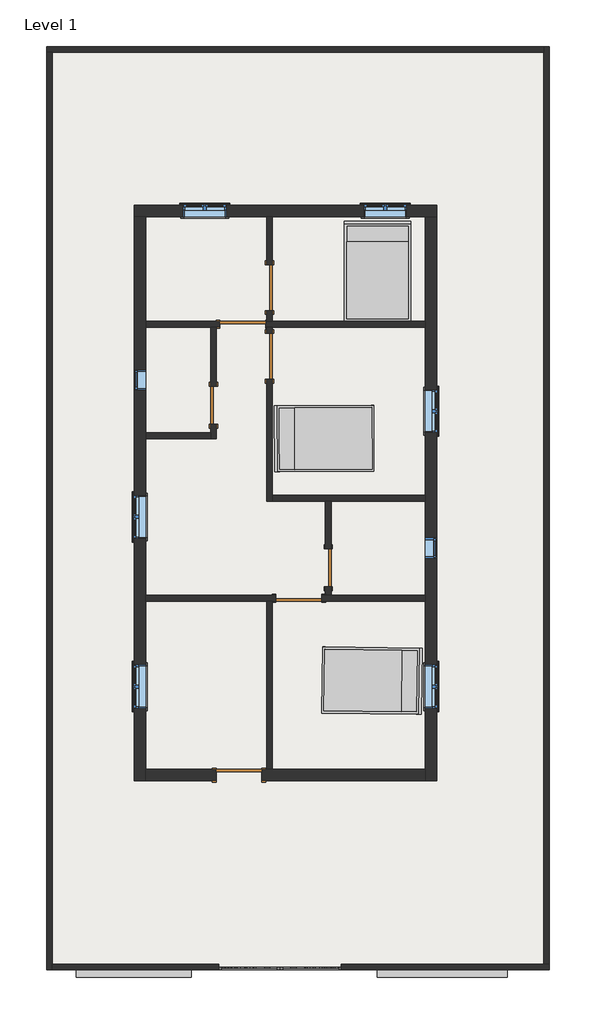
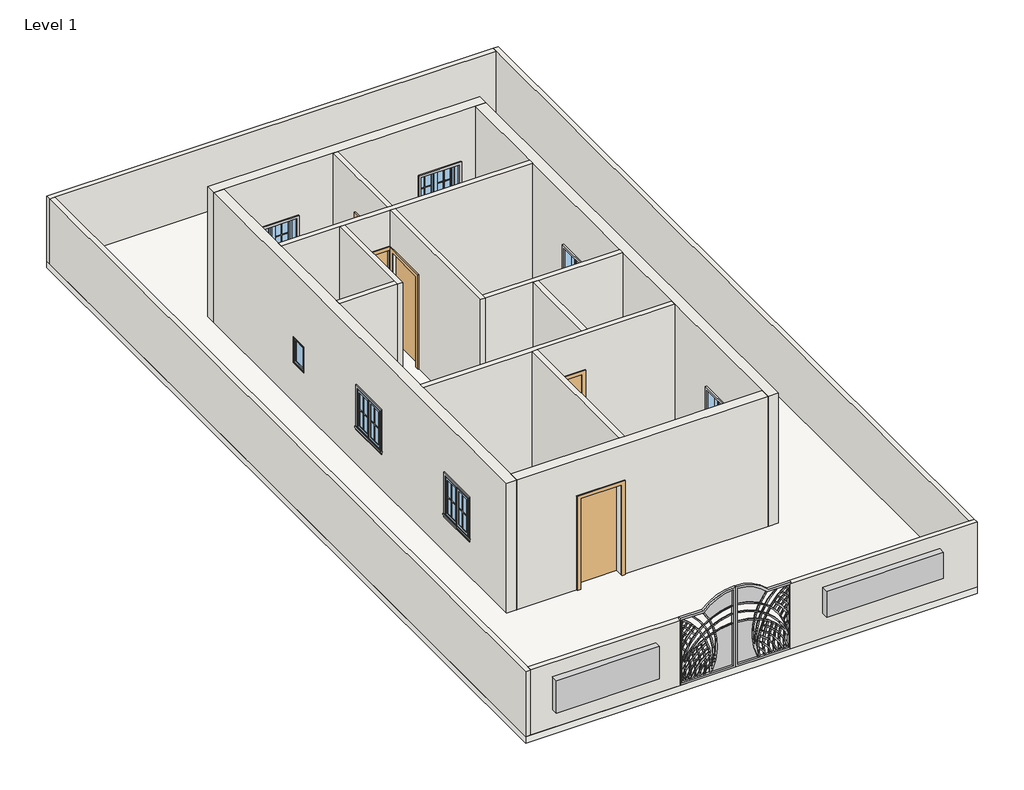
# One storey, incomplete: 26 proxies, 17 walls, 8 windows, 7 doors, 3 furniture elements, 1 slab.
"""IFC4 building model written with IfcOpenShell, lengths in millimetres."""

from ifc_helpers import new_model, si_unit, frame, origin, origin_with_axes, place, context, project, spatial, polyline, outline, extrude, faceted_brep, transform, mapped, element, save
from components import generic_models_6bc30956, generic_models_1_generic_models_1_74e75cdd, muntin_pattern_2x2_muntin_pattern_2x2_b3fe6957, muntin_pattern_2x2_muntin_pattern_2x2_3e0ecaf2, trim_window_exterior_flat_with_sill_41619996, trim_window_interior_flat_picture_frame_51c85655, door_d8f5dbb5, door_f2b275c1, door_e5f9f3c4, door_305aa2a5, door_0ca8825f, bed_17739_bed_17739_15c61121, window_aa618e30, window_339605e1

model = new_model("IFC4")

# Units and contexts
model_context = context("Model", 3, world=origin())
ifc_project = project(units=[si_unit("LENGTHUNIT", "METRE", prefix="MILLI")], contexts=[model_context])

# Site, building, storey
site = spatial("IfcSite", under=ifc_project)
building = spatial("IfcBuilding", under=site)
storey = spatial("IfcBuildingStorey", under=building, Name="Level 1", Elevation=0.0)

# Proxies
placement = place(None, origin())
generic_models_shape = generic_models_6bc30956(model_context)
element("IfcBuildingElementProxy", 1, Name="Generic Models", at=placement, inside=storey, context=model_context, shape_type="MappedRepresentation", body=[
    mapped(generic_models_shape, transform((-1369.5415084, -8760.8383207, 0.0), x_axis=(1.0, 0.0, 0.0), y_axis=(0.0, 1.0, 0.0), z_axis=(0.0, 0.0, 1.0))),
])
generic_models_1_generic_models_1_shape = generic_models_1_generic_models_1_74e75cdd(model_context)
element("IfcBuildingElementProxy", 2, Name="Generic Models 1 : Generic Models 1", ObjectType="Generic Models 1 : Generic Models 1", at=placement, inside=storey, context=model_context, shape_type="MappedRepresentation", body=[
    mapped(generic_models_1_generic_models_1_shape, transform((0.0, 0.0, 0.0), x_axis=(1.0, 0.0, 0.0), y_axis=(0.0, 1.0, 0.0), z_axis=(0.0, 0.0, 1.0))),
])
muntin_pattern_2x2_muntin_pattern_2x2_shape = muntin_pattern_2x2_muntin_pattern_2x2_b3fe6957(model_context)
element("IfcBuildingElementProxy", 3, Name="Muntin Pattern_2x2 : Muntin Pattern_2x2", ObjectType="Muntin Pattern_2x2 : Muntin Pattern_2x2", at=placement, inside=storey, context=model_context, shape_type="MappedRepresentation", body=[
    mapped(muntin_pattern_2x2_muntin_pattern_2x2_shape, transform((517.9959916, 6415.1185985, 984.25), x_axis=(1.0, 0.0, 0.0), y_axis=(0.0, 1.0, 0.0), z_axis=(0.0, 0.0, 1.0))),
])
element("IfcBuildingElementProxy", 4, Name="Muntin Pattern_2x2 : Muntin Pattern_2x2", ObjectType="Muntin Pattern_2x2 : Muntin Pattern_2x2", at=placement, inside=storey, context=model_context, shape_type="MappedRepresentation", body=[
    mapped(muntin_pattern_2x2_muntin_pattern_2x2_shape, transform((-3079.2790084, 6415.1185985, 984.25), x_axis=(1.0, 0.0, 0.0), y_axis=(0.0, 1.0, 0.0), z_axis=(0.0, 0.0, 1.0))),
])
element("IfcBuildingElementProxy", 5, Name="Muntin Pattern_2x2 : Muntin Pattern_2x2", ObjectType="Muntin Pattern_2x2 : Muntin Pattern_2x2", at=placement, inside=storey, context=model_context, shape_type="MappedRepresentation", body=[
    mapped(muntin_pattern_2x2_muntin_pattern_2x2_shape, transform((1751.4834916, 2536.8560985, 984.25), x_axis=(0.0, -1.0, 0.0), y_axis=(1.0, 0.0, 0.0), z_axis=(0.0, 0.0, 1.0))),
])
element("IfcBuildingElementProxy", 6, Name="Muntin Pattern_2x2 : Muntin Pattern_2x2", ObjectType="Muntin Pattern_2x2 : Muntin Pattern_2x2", at=placement, inside=storey, context=model_context, shape_type="MappedRepresentation", body=[
    mapped(muntin_pattern_2x2_muntin_pattern_2x2_shape, transform((-4261.9665084, 0.0310985, 984.25), x_axis=(0.0, 1.0, 0.0), y_axis=(-1.0, 0.0, 0.0), z_axis=(0.0, 0.0, 1.0))),
])
element("IfcBuildingElementProxy", 7, Name="Muntin Pattern_2x2 : Muntin Pattern_2x2", ObjectType="Muntin Pattern_2x2 : Muntin Pattern_2x2", at=placement, inside=storey, context=model_context, shape_type="MappedRepresentation", body=[
    mapped(muntin_pattern_2x2_muntin_pattern_2x2_shape, transform((-4261.9665084, -3381.3439015, 984.25), x_axis=(0.0, 1.0, 0.0), y_axis=(-1.0, 0.0, 0.0), z_axis=(0.0, 0.0, 1.0))),
])
element("IfcBuildingElementProxy", 8, Name="Muntin Pattern_2x2 : Muntin Pattern_2x2", ObjectType="Muntin Pattern_2x2 : Muntin Pattern_2x2", at=placement, inside=storey, context=model_context, shape_type="MappedRepresentation", body=[
    mapped(muntin_pattern_2x2_muntin_pattern_2x2_shape, transform((1751.4834916, -2952.7189015, 984.25), x_axis=(0.0, -1.0, 0.0), y_axis=(1.0, 0.0, 0.0), z_axis=(0.0, 0.0, 1.0))),
])
muntin_pattern_2x2_muntin_pattern_2x2_2_shape = muntin_pattern_2x2_muntin_pattern_2x2_3e0ecaf2(model_context)
element("IfcBuildingElementProxy", 9, Name="Muntin Pattern_2x2 : Muntin Pattern_2x2", ObjectType="Muntin Pattern_2x2 : Muntin Pattern_2x2", at=placement, inside=storey, context=model_context, shape_type="MappedRepresentation", body=[
    mapped(muntin_pattern_2x2_muntin_pattern_2x2_2_shape, transform((946.6209916, 6415.1185985, 984.25), x_axis=(-1.0, 0.0, 0.0), y_axis=(0.0, -1.0, 0.0), z_axis=(0.0, 0.0, 1.0))),
])
element("IfcBuildingElementProxy", 10, Name="Muntin Pattern_2x2 : Muntin Pattern_2x2", ObjectType="Muntin Pattern_2x2 : Muntin Pattern_2x2", at=placement, inside=storey, context=model_context, shape_type="MappedRepresentation", body=[
    mapped(muntin_pattern_2x2_muntin_pattern_2x2_2_shape, transform((-2650.6540084, 6415.1185985, 984.25), x_axis=(-1.0, 0.0, 0.0), y_axis=(0.0, -1.0, 0.0), z_axis=(0.0, 0.0, 1.0))),
])
element("IfcBuildingElementProxy", 11, Name="Muntin Pattern_2x2 : Muntin Pattern_2x2", ObjectType="Muntin Pattern_2x2 : Muntin Pattern_2x2", at=placement, inside=storey, context=model_context, shape_type="MappedRepresentation", body=[
    mapped(muntin_pattern_2x2_muntin_pattern_2x2_2_shape, transform((1751.4834916, 2108.2310985, 984.25), x_axis=(0.0, 1.0, 0.0), y_axis=(-1.0, 0.0, 0.0), z_axis=(0.0, 0.0, 1.0))),
])
element("IfcBuildingElementProxy", 12, Name="Muntin Pattern_2x2 : Muntin Pattern_2x2", ObjectType="Muntin Pattern_2x2 : Muntin Pattern_2x2", at=placement, inside=storey, context=model_context, shape_type="MappedRepresentation", body=[
    mapped(muntin_pattern_2x2_muntin_pattern_2x2_2_shape, transform((-4261.9665084, 428.6560985, 984.25), x_axis=(0.0, -1.0, 0.0), y_axis=(1.0, 0.0, 0.0), z_axis=(0.0, 0.0, 1.0))),
])
element("IfcBuildingElementProxy", 13, Name="Muntin Pattern_2x2 : Muntin Pattern_2x2", ObjectType="Muntin Pattern_2x2 : Muntin Pattern_2x2", at=placement, inside=storey, context=model_context, shape_type="MappedRepresentation", body=[
    mapped(muntin_pattern_2x2_muntin_pattern_2x2_2_shape, transform((-4261.9665084, -2952.7189015, 984.25), x_axis=(0.0, -1.0, 0.0), y_axis=(1.0, 0.0, 0.0), z_axis=(0.0, 0.0, 1.0))),
])
element("IfcBuildingElementProxy", 14, Name="Muntin Pattern_2x2 : Muntin Pattern_2x2", ObjectType="Muntin Pattern_2x2 : Muntin Pattern_2x2", at=placement, inside=storey, context=model_context, shape_type="MappedRepresentation", body=[
    mapped(muntin_pattern_2x2_muntin_pattern_2x2_2_shape, transform((1751.4834916, -3381.3439015, 984.25), x_axis=(0.0, 1.0, 0.0), y_axis=(-1.0, 0.0, 0.0), z_axis=(0.0, 0.0, 1.0))),
])
trim_window_exterior_flat_with_sill_shape = trim_window_exterior_flat_with_sill_41619996(model_context)
element("IfcBuildingElementProxy", 15, Name="Trim-Window-Exterior-Flat : with Sill", ObjectType="Trim-Window-Exterior-Flat : with Sill", at=placement, inside=storey, context=model_context, shape_type="MappedRepresentation", body=[
    mapped(trim_window_exterior_flat_with_sill_shape, transform((732.3084916, 6424.6435985, 1828.8), x_axis=(-1.0, 0.0, 0.0), y_axis=(0.0, 0.0, 1.0), z_axis=(0.0, 1.0, 0.0))),
])
element("IfcBuildingElementProxy", 16, Name="Trim-Window-Exterior-Flat : with Sill", ObjectType="Trim-Window-Exterior-Flat : with Sill", at=placement, inside=storey, context=model_context, shape_type="MappedRepresentation", body=[
    mapped(trim_window_exterior_flat_with_sill_shape, transform((-2864.9665084, 6424.6435985, 1828.8), x_axis=(-1.0, 0.0, 0.0), y_axis=(0.0, 0.0, 1.0), z_axis=(0.0, 1.0, 0.0))),
])
element("IfcBuildingElementProxy", 17, Name="Trim-Window-Exterior-Flat : with Sill", ObjectType="Trim-Window-Exterior-Flat : with Sill", at=placement, inside=storey, context=model_context, shape_type="MappedRepresentation", body=[
    mapped(trim_window_exterior_flat_with_sill_shape, transform((1761.0084916, 2322.5435985, 1828.8), x_axis=(0.0, 1.0, 0.0), y_axis=(0.0, 0.0, 1.0), z_axis=(1.0, 0.0, 0.0))),
])
element("IfcBuildingElementProxy", 18, Name="Trim-Window-Exterior-Flat : with Sill", ObjectType="Trim-Window-Exterior-Flat : with Sill", at=placement, inside=storey, context=model_context, shape_type="MappedRepresentation", body=[
    mapped(trim_window_exterior_flat_with_sill_shape, transform((-4271.4915084, 214.3435985, 1828.8), x_axis=(0.0, -1.0, 0.0), y_axis=(0.0, 0.0, 1.0), z_axis=(-1.0, 0.0, 0.0))),
])
element("IfcBuildingElementProxy", 19, Name="Trim-Window-Exterior-Flat : with Sill", ObjectType="Trim-Window-Exterior-Flat : with Sill", at=placement, inside=storey, context=model_context, shape_type="MappedRepresentation", body=[
    mapped(trim_window_exterior_flat_with_sill_shape, transform((-4271.4915084, -3167.0314015, 1828.8), x_axis=(0.0, -1.0, 0.0), y_axis=(0.0, 0.0, 1.0), z_axis=(-1.0, 0.0, 0.0))),
])
element("IfcBuildingElementProxy", 20, Name="Trim-Window-Exterior-Flat : with Sill", ObjectType="Trim-Window-Exterior-Flat : with Sill", at=placement, inside=storey, context=model_context, shape_type="MappedRepresentation", body=[
    mapped(trim_window_exterior_flat_with_sill_shape, transform((1761.0084916, -3167.0314015, 1828.8), x_axis=(0.0, 1.0, 0.0), y_axis=(0.0, 0.0, 1.0), z_axis=(1.0, 0.0, 0.0))),
])
trim_window_interior_flat_picture_frame_shape = trim_window_interior_flat_picture_frame_51c85655(model_context)
element("IfcBuildingElementProxy", 21, Name="Trim-Window-Interior-Flat : Picture Frame", ObjectType="Trim-Window-Interior-Flat : Picture Frame", at=placement, inside=storey, context=model_context, shape_type="MappedRepresentation", body=[
    mapped(trim_window_interior_flat_picture_frame_shape, transform((732.3084916, 6196.0435985, 1828.8), x_axis=(1.0, 0.0, 0.0), y_axis=(0.0, 0.0, 1.0), z_axis=(0.0, -1.0, 0.0))),
])
element("IfcBuildingElementProxy", 22, Name="Trim-Window-Interior-Flat : Picture Frame", ObjectType="Trim-Window-Interior-Flat : Picture Frame", at=placement, inside=storey, context=model_context, shape_type="MappedRepresentation", body=[
    mapped(trim_window_interior_flat_picture_frame_shape, transform((-2864.9665084, 6196.0435985, 1828.8), x_axis=(1.0, 0.0, 0.0), y_axis=(0.0, 0.0, 1.0), z_axis=(0.0, -1.0, 0.0))),
])
element("IfcBuildingElementProxy", 23, Name="Trim-Window-Interior-Flat : Picture Frame", ObjectType="Trim-Window-Interior-Flat : Picture Frame", at=placement, inside=storey, context=model_context, shape_type="MappedRepresentation", body=[
    mapped(trim_window_interior_flat_picture_frame_shape, transform((1532.4084916, 2322.5435985, 1828.8), x_axis=(0.0, -1.0, 0.0), y_axis=(0.0, 0.0, 1.0), z_axis=(-1.0, 0.0, 0.0))),
])
element("IfcBuildingElementProxy", 24, Name="Trim-Window-Interior-Flat : Picture Frame", ObjectType="Trim-Window-Interior-Flat : Picture Frame", at=placement, inside=storey, context=model_context, shape_type="MappedRepresentation", body=[
    mapped(trim_window_interior_flat_picture_frame_shape, transform((-4042.8915084, 214.3435985, 1828.8), x_axis=(0.0, 1.0, 0.0), y_axis=(0.0, 0.0, 1.0), z_axis=(1.0, 0.0, 0.0))),
])
element("IfcBuildingElementProxy", 25, Name="Trim-Window-Interior-Flat : Picture Frame", ObjectType="Trim-Window-Interior-Flat : Picture Frame", at=placement, inside=storey, context=model_context, shape_type="MappedRepresentation", body=[
    mapped(trim_window_interior_flat_picture_frame_shape, transform((-4042.8915084, -3167.0314015, 1828.8), x_axis=(0.0, 1.0, 0.0), y_axis=(0.0, 0.0, 1.0), z_axis=(1.0, 0.0, 0.0))),
])
element("IfcBuildingElementProxy", 26, Name="Trim-Window-Interior-Flat : Picture Frame", ObjectType="Trim-Window-Interior-Flat : Picture Frame", at=placement, inside=storey, context=model_context, shape_type="MappedRepresentation", body=[
    mapped(trim_window_interior_flat_picture_frame_shape, transform((1532.4084916, -3167.0314015, 1828.8), x_axis=(0.0, -1.0, 0.0), y_axis=(0.0, 0.0, 1.0), z_axis=(-1.0, 0.0, 0.0))),
])

# Doors
door_shape = door_d8f5dbb5(model_context)
element("IfcDoor", 27, ObjectType="Single-Flush : 30\" x 80\"", at=placement, inside=storey, context=model_context, shape_type="MappedRepresentation", body=[
    mapped(door_shape, transform((-404.3415084, -795.3064015, 0.0), x_axis=(0.0, -1.0, 0.0), y_axis=(1.0, 0.0, 0.0), z_axis=(0.0, 0.0, 1.0))),
])
door_2_shape = door_f2b275c1(model_context)
element("IfcDoor", 28, ObjectType="Single-Flush : 30\" x 80\"", at=placement, inside=storey, context=model_context, shape_type="MappedRepresentation", body=[
    mapped(door_2_shape, transform((-2690.3415084, 2443.1935985, 0.0), x_axis=(0.0, -1.0, 0.0), y_axis=(1.0, 0.0, 0.0), z_axis=(0.0, 0.0, 1.0))),
])
door_3_shape = door_e5f9f3c4(model_context)
element("IfcDoor", 29, ObjectType="Single-Flush : 36\" x 84\"", at=placement, inside=storey, context=model_context, shape_type="MappedRepresentation", body=[
    mapped(door_3_shape, transform((-2106.1415084, 4056.0935985, 0.0), x_axis=(1.0, 0.0, 0.0), y_axis=(0.0, 1.0, 0.0), z_axis=(0.0, 0.0, 1.0))),
])
element("IfcDoor", 30, ObjectType="Single-Flush : 36\" x 84\"", at=placement, inside=storey, context=model_context, shape_type="MappedRepresentation", body=[
    mapped(door_3_shape, transform((-1572.7415084, 4786.3435985, 0.0), x_axis=(0.0, -1.0, 0.0), y_axis=(1.0, 0.0, 0.0), z_axis=(0.0, 0.0, 1.0))),
])
element("IfcDoor", 31, ObjectType="Single-Flush : 36\" x 84\"", at=placement, inside=storey, context=model_context, shape_type="MappedRepresentation", body=[
    mapped(door_3_shape, transform((-988.5415084, -1404.9064015, 0.0), x_axis=(-1.0, 0.0, 0.0), y_axis=(0.0, -1.0, 0.0), z_axis=(0.0, 0.0, 1.0))),
])
door_4_shape = door_305aa2a5(model_context)
element("IfcDoor", 32, ObjectType="Single-Flush : 36\" x 84\"", at=placement, inside=storey, context=model_context, shape_type="MappedRepresentation", body=[
    mapped(door_4_shape, transform((-1572.7415084, 3414.7435985, 0.0), x_axis=(0.0, 1.0, 0.0), y_axis=(-1.0, 0.0, 0.0), z_axis=(0.0, 0.0, 1.0))),
])
door_5_shape = door_0ca8825f(model_context)
element("IfcDoor", 33, ObjectType="Single-Flush : 36\" x 84\"", at=placement, inside=storey, context=model_context, shape_type="MappedRepresentation", body=[
    mapped(door_5_shape, transform((-2182.3415084, -4929.1564015, 0.0), x_axis=(1.0, 0.0, 0.0), y_axis=(0.0, 1.0, 0.0), z_axis=(0.0, 0.0, 1.0))),
])

# Furniture
bed_17739_bed_17739_shape = bed_17739_bed_17739_15c61121(model_context)
element("IfcFurniture", 34, ObjectType="Bed_17739 : Bed_17739", at=placement, inside=storey, context=model_context, shape_type="MappedRepresentation", body=[
    mapped(bed_17739_bed_17739_shape, transform((579.9084916, 5091.1435985, 0.0), x_axis=(1.0, 0.0, 0.0), y_axis=(0.0, 1.0, 0.0), z_axis=(0.0, 0.0, 1.0))),
])
element("IfcFurniture", 35, ObjectType="Bed_17739 : Bed_17739", at=placement, inside=storey, context=model_context, shape_type="MappedRepresentation", body=[
    mapped(bed_17739_bed_17739_shape, transform((-461.4915084, 1776.4435985, 0.0), x_axis=(-0.00529598194226197, 0.9999859761893001, 0.0), y_axis=(-0.9999859761893001, -0.00529598194226197, 0.0), z_axis=(0.0, 0.0, 1.0))),
])
element("IfcFurniture", 36, ObjectType="Bed_17739 : Bed_17739", at=placement, inside=storey, context=model_context, shape_type="MappedRepresentation", body=[
    mapped(bed_17739_bed_17739_shape, transform((445.2457081, -3048.1973462, 0.0), x_axis=(-0.012781947661401841, -0.9999183075701641, 0.0), y_axis=(0.9999183075701641, -0.012781947661401841, 0.0), z_axis=(0.0, 0.0, 1.0))),
])

# Slab
element("IfcSlab", 37, ObjectType="Generic - 12\"", at=placement, inside=storey, context=model_context, shape_type="SweptSolid", body=[
    extrude(outline(polyline([(4001.9228037, 9590.6616793), (4001.9228037, -8811.6383207), (-6018.3771963, -8811.6383207), (-6018.3771963, 9590.6616793), (4001.9228037, 9590.6616793)])), frame((0.0, 0.0, -152.4), z_axis=(0.0, 0.0, 1.0), x_axis=(1.0, 0.0, 0.0)), (0.0, 0.0, 1.0), 152.4),
])

# Walls
element("IfcWall", 38, ObjectType="WALL4.5\"", at=placement, inside=storey, context=model_context, shape_type="Brep", body=[
    faceted_brep([(-1648.9415084, 3998.9435985, 2133.6), (-1648.9415084, 3998.9435985, 0.0), (-1629.8915084, 3998.9435985, 0.0), (-1515.5915084, 3998.9435985, 0.0), (1532.4084916, 3998.9435985, 0.0), (1532.4084916, 3998.9435985, 3048.0), (-1515.5915084, 3998.9435985, 3048.0), (-1629.8915084, 3998.9435985, 3048.0), (-2633.1915084, 3998.9435985, 3048.0), (-2747.4915084, 3998.9435985, 3048.0), (-4042.8915084, 3998.9435985, 3048.0), (-4042.8915084, 3998.9435985, 0.0), (-2747.4915084, 3998.9435985, 0.0), (-2633.1915084, 3998.9435985, 0.0), (-2563.3415084, 3998.9435985, 0.0), (-2563.3415084, 3998.9435985, 2133.6), (1532.4084916, 4113.2435985, 0.0), (-1515.5915084, 4113.2435985, 0.0), (-1629.8915084, 4113.2435985, 0.0), (-1648.9415084, 4113.2435985, 0.0), (-1648.9415084, 4113.2435985, 2133.6), (-2563.3415084, 4113.2435985, 2133.6), (-2563.3415084, 4113.2435985, 0.0), (-4042.8915084, 4113.2435985, 0.0), (-4042.8915084, 4113.2435985, 3048.0), (-1629.8915084, 4113.2435985, 3048.0), (-1515.5915084, 4113.2435985, 3048.0), (1532.4084916, 4113.2435985, 3048.0)], [[[0, 1, 2, 3, 4, 5, 6, 7, 8, 9, 10, 11, 12, 13, 14, 15]], [[16, 17, 18, 19, 20, 21, 22, 23, 24, 25, 26, 27]], [[4, 3, 2, 1, 19, 18, 17, 16]], [[14, 13, 12, 11, 23, 22]], [[5, 4, 16, 27]], [[11, 10, 24, 23]], [[20, 19, 1, 0]], [[21, 20, 0, 15]], [[22, 21, 15, 14]], [[10, 9, 8, 7, 6, 5, 27, 26, 25, 24]]]),
])
element("IfcWall", 39, ObjectType="WALL4.5\"", at=placement, inside=storey, context=model_context, shape_type="Brep", body=[
    faceted_brep([(-1629.8915084, 6196.0435985, 3048.0), (-1629.8915084, 6196.0435985, 0.0), (-1629.8915084, 5243.5435985, 0.0), (-1629.8915084, 5243.5435985, 2133.6), (-1629.8915084, 4329.1435985, 2133.6), (-1629.8915084, 4329.1435985, 0.0), (-1629.8915084, 4113.2435985, 0.0), (-1629.8915084, 4113.2435985, 3048.0), (-1515.5915084, 6196.0435985, 0.0), (-1515.5915084, 6196.0435985, 3048.0), (-1515.5915084, 4113.2435985, 3048.0), (-1515.5915084, 4113.2435985, 0.0), (-1515.5915084, 4329.1435985, 0.0), (-1515.5915084, 4329.1435985, 2133.6), (-1515.5915084, 5243.5435985, 2133.6), (-1515.5915084, 5243.5435985, 0.0)], [[[0, 1, 2, 3, 4, 5, 6, 7]], [[8, 9, 10, 11, 12, 13, 14, 15]], [[1, 8, 15, 2]], [[5, 12, 11, 6]], [[1, 0, 9, 8]], [[7, 6, 11, 10]], [[13, 12, 5, 4]], [[14, 13, 4, 3]], [[15, 14, 3, 2]], [[9, 0, 7, 10]]]),
    faceted_brep([(-1629.8915084, 531.8435985, 0.0), (-1629.8915084, 531.8435985, 3048.0), (-1629.8915084, 3998.9435985, 3048.0), (-1629.8915084, 3998.9435985, 0.0), (-1629.8915084, 3871.9435985, 0.0), (-1629.8915084, 3871.9435985, 2133.6), (-1629.8915084, 2957.5435985, 2133.6), (-1629.8915084, 2957.5435985, 0.0), (-1515.5915084, 531.8435985, 3048.0), (-1515.5915084, 531.8435985, 0.0), (-1515.5915084, 646.1435985, 0.0), (-1515.5915084, 2957.5435985, 0.0), (-1515.5915084, 2957.5435985, 2133.6), (-1515.5915084, 3871.9435985, 2133.6), (-1515.5915084, 3871.9435985, 0.0), (-1515.5915084, 3998.9435985, 0.0), (-1515.5915084, 3998.9435985, 3048.0), (-1515.5915084, 646.1435985, 3048.0)], [[[0, 1, 2, 3, 4, 5, 6, 7]], [[8, 9, 10, 11, 12, 13, 14, 15, 16, 17]], [[9, 0, 7, 11, 10]], [[14, 4, 3, 15]], [[3, 2, 16, 15]], [[1, 0, 9, 8]], [[5, 4, 14, 13]], [[6, 5, 13, 12]], [[7, 6, 12, 11]], [[1, 8, 17, 16, 2]]]),
])
element("IfcWall", 40, ObjectType="WALL4.5\"", at=placement, inside=storey, context=model_context, shape_type="Brep", body=[
    faceted_brep([(-1515.5915084, 531.8435985, 0.0), (-461.4915084, 531.8435985, 0.0), (-347.1915084, 531.8435985, 0.0), (1532.4084916, 531.8435985, 0.0), (1532.4084916, 531.8435985, 3048.0), (-347.1915084, 531.8435985, 3048.0), (-461.4915084, 531.8435985, 3048.0), (-1515.5915084, 531.8435985, 3048.0), (-1515.5915084, 646.1435985, 0.0), (-1515.5915084, 646.1435985, 3048.0), (1532.4084916, 646.1435985, 3048.0), (1532.4084916, 646.1435985, 0.0)], [[[0, 1, 2, 3, 4, 5, 6, 7]], [[8, 9, 10, 11]], [[3, 2, 1, 0, 8, 11]], [[0, 7, 9, 8]], [[4, 3, 11, 10]], [[7, 6, 5, 4, 10, 9]]]),
])
element("IfcWall", 41, ObjectType="WALL4.5\"", at=placement, inside=storey, context=model_context, shape_type="Brep", body=[
    faceted_brep([(-2747.4915084, 2062.1935985, 2032.0), (-2747.4915084, 2062.1935985, 0.0), (-2747.4915084, 1890.7435985, 0.0), (-2747.4915084, 1776.4435985, 0.0), (-2747.4915084, 1776.4435985, 3048.0), (-2747.4915084, 1890.7435985, 3048.0), (-2747.4915084, 3998.9435985, 3048.0), (-2747.4915084, 3998.9435985, 0.0), (-2747.4915084, 2824.1935985, 0.0), (-2747.4915084, 2824.1935985, 2032.0), (-2633.1915084, 1776.4435985, 0.0), (-2633.1915084, 2062.1935985, 0.0), (-2633.1915084, 2062.1935985, 2032.0), (-2633.1915084, 2824.1935985, 2032.0), (-2633.1915084, 2824.1935985, 0.0), (-2633.1915084, 3998.9435985, 0.0), (-2633.1915084, 3998.9435985, 3048.0), (-2633.1915084, 1776.4435985, 3048.0)], [[[0, 1, 2, 3, 4, 5, 6, 7, 8, 9]], [[10, 11, 12, 13, 14, 15, 16, 17]], [[8, 7, 15, 14]], [[3, 2, 1, 11, 10]], [[7, 6, 16, 15]], [[4, 3, 10, 17]], [[12, 11, 1, 0]], [[13, 12, 0, 9]], [[14, 13, 9, 8]], [[6, 5, 4, 17, 16]]]),
])
element("IfcWall", 42, ObjectType="WALL4.5\"", at=placement, inside=storey, context=model_context, shape_type="SweptSolid", body=[
    extrude(outline(polyline([(-2747.4915084, 1776.4435985), (-4042.8915084, 1776.4435985), (-4042.8915084, 1890.7435985), (-2747.4915084, 1890.7435985), (-2747.4915084, 1776.4435985)])), origin_with_axes(), (0.0, 0.0, 1.0), 3048.0),
])
element("IfcWall", 43, ObjectType="WALL4.5\"", at=placement, inside=storey, context=model_context, shape_type="SweptSolid", body=[
    extrude(outline(polyline([(-1176.3064015, 2032.0), (-1176.3064015, 0.0), (-1347.7564015, 0.0), (-1347.7564015, 3048.0), (531.8435985, 3048.0), (531.8435985, 0.0), (-414.3064015, 0.0), (-414.3064015, 2032.0), (-1176.3064015, 2032.0)])), frame((-461.4915084, 0.0, 0.0), z_axis=(1.0, 0.0, 0.0), x_axis=(0.0, 1.0, 0.0)), (0.0, 0.0, 1.0), 114.3),
])
element("IfcWall", 44, ObjectType="WALL4.5\"", at=placement, inside=storey, context=model_context, shape_type="Brep", body=[
    faceted_brep([(-4042.8915084, -1462.0564015, 0.0), (-1629.8915084, -1462.0564015, 0.0), (-1515.5915084, -1462.0564015, 0.0), (-1445.7415084, -1462.0564015, 0.0), (-1445.7415084, -1462.0564015, 2133.6), (-531.3415084, -1462.0564015, 2133.6), (-531.3415084, -1462.0564015, 0.0), (1532.4084916, -1462.0564015, 0.0), (1532.4084916, -1462.0564015, 3048.0), (-1515.5915084, -1462.0564015, 3048.0), (-1629.8915084, -1462.0564015, 3048.0), (-4042.8915084, -1462.0564015, 3048.0), (-1445.7415084, -1347.7564015, 2133.6), (-1445.7415084, -1347.7564015, 0.0), (-4042.8915084, -1347.7564015, 0.0), (-4042.8915084, -1347.7564015, 3048.0), (-461.4915084, -1347.7564015, 3048.0), (-347.1915084, -1347.7564015, 3048.0), (1532.4084916, -1347.7564015, 3048.0), (1532.4084916, -1347.7564015, 0.0), (-347.1915084, -1347.7564015, 0.0), (-461.4915084, -1347.7564015, 0.0), (-531.3415084, -1347.7564015, 0.0), (-531.3415084, -1347.7564015, 2133.6)], [[[0, 1, 2, 3, 4, 5, 6, 7, 8, 9, 10, 11]], [[12, 13, 14, 15, 16, 17, 18, 19, 20, 21, 22, 23]], [[14, 13, 3, 2, 1, 0]], [[22, 21, 20, 19, 7, 6]], [[8, 7, 19, 18]], [[0, 11, 15, 14]], [[4, 3, 13, 12]], [[5, 4, 12, 23]], [[6, 5, 23, 22]], [[11, 10, 9, 8, 18, 17, 16, 15]]]),
])
element("IfcWall", 45, ObjectType="WALL4.5\"", at=placement, inside=storey, context=model_context, shape_type="SweptSolid", body=[
    extrude(outline(polyline([(-1629.8915084, -4814.8564015), (-1629.8915084, -1462.0564015), (-1515.5915084, -1462.0564015), (-1515.5915084, -4814.8564015), (-1629.8915084, -4814.8564015)])), origin_with_axes(), (0.0, 0.0, 1.0), 3048.0),
])
element("IfcWall", 46, ObjectType="WALL4.5\"", at=placement, inside=storey, context=model_context, shape_type="Brep", body=[
    faceted_brep([(-6018.3771963, 9476.3616793, 0.0), (-5904.0771963, 9476.3616793, 0.0), (3887.6228037, 9476.3616793, 0.0), (3887.6228037, 9476.3616793, 1524.0), (-5904.0771963, 9476.3616793, 1524.0), (-6018.3771963, 9476.3616793, 1524.0), (-6018.3771963, 9590.6616793, 0.0), (-6018.3771963, 9590.6616793, 1524.0), (3887.6228037, 9590.6616793, 1524.0), (3887.6228037, 9590.6616793, 0.0)], [[[0, 1, 2, 3, 4, 5]], [[6, 7, 8, 9]], [[2, 1, 0, 6, 9]], [[5, 4, 3, 8, 7]], [[0, 5, 7, 6]], [[3, 2, 9, 8]]]),
])
element("IfcWall", 47, ObjectType="WALL4.5\"", at=placement, inside=storey, context=model_context, shape_type="Brep", body=[
    faceted_brep([(-5904.0771963, -8811.6383207, 0.0), (-5904.0771963, -8697.3383207, 0.0), (-5904.0771963, 9476.3616793, 0.0), (-5904.0771963, 9476.3616793, 1524.0), (-5904.0771963, -8697.3383207, 1524.0), (-5904.0771963, -8811.6383207, 1524.0), (-6018.3771963, -8811.6383207, 0.0), (-6018.3771963, -8811.6383207, 1524.0), (-6018.3771963, 9476.3616793, 1524.0), (-6018.3771963, 9476.3616793, 0.0)], [[[0, 1, 2, 3, 4, 5]], [[6, 7, 8, 9]], [[2, 1, 0, 6, 9]], [[5, 4, 3, 8, 7]], [[0, 5, 7, 6]], [[3, 2, 9, 8]]]),
])
element("IfcWall", 48, ObjectType="WALL4.5\"", at=placement, inside=storey, context=model_context, shape_type="Brep", body=[
    faceted_brep([(4001.9228037, -8697.3383207, 0.0), (3887.6228037, -8697.3383207, 0.0), (-144.6271963, -8697.3383207, 0.0), (-144.6271963, -8697.3383207, 1524.0), (3887.6228037, -8697.3383207, 1524.0), (4001.9228037, -8697.3383207, 1524.0), (4001.9228037, -8811.6383207, 0.0), (4001.9228037, -8811.6383207, 1524.0), (-144.6271963, -8811.6383207, 1524.0), (-144.6271963, -8811.6383207, 0.0)], [[[0, 1, 2, 3, 4, 5]], [[6, 7, 8, 9]], [[2, 1, 0, 6, 9]], [[3, 2, 9, 8]], [[5, 4, 3, 8, 7]], [[0, 5, 7, 6]]]),
])
element("IfcWall", 49, ObjectType="WALL4.5\"", at=placement, inside=storey, context=model_context, shape_type="Brep", body=[
    faceted_brep([(3887.6228037, 9590.6616793, 0.0), (3887.6228037, 9476.3616793, 0.0), (3887.6228037, -8697.3383207, 0.0), (3887.6228037, -8697.3383207, 1524.0), (3887.6228037, 9476.3616793, 1524.0), (3887.6228037, 9590.6616793, 1524.0), (4001.9228037, 9590.6616793, 0.0), (4001.9228037, 9590.6616793, 1524.0), (4001.9228037, -8697.3383207, 1524.0), (4001.9228037, -8697.3383207, 0.0)], [[[0, 1, 2, 3, 4, 5]], [[6, 7, 8, 9]], [[2, 1, 0, 6, 9]], [[5, 4, 3, 8, 7]], [[0, 5, 7, 6]], [[3, 2, 9, 8]]]),
])
element("IfcWall", 50, ObjectType="WALL4.5\"", at=placement, inside=storey, context=model_context, shape_type="SweptSolid", body=[
    extrude(outline(polyline([(-5904.0771963, -8697.3383207), (-2583.0271963, -8697.3383207), (-2583.0271963, -8811.6383207), (-5904.0771963, -8811.6383207), (-5904.0771963, -8697.3383207)])), origin_with_axes(), (0.0, 0.0, 1.0), 1524.0),
])
element("IfcWall", 51, ObjectType="WALL9\"", at=placement, inside=storey, context=model_context, shape_type="Brep", body=[
    faceted_brep([(-4271.4915084, 6196.0435985, 0.0), (-4042.8915084, 6196.0435985, 0.0), (-1629.8915084, 6196.0435985, 0.0), (-1515.5915084, 6196.0435985, 0.0), (1532.4084916, 6196.0435985, 0.0), (1761.0084916, 6196.0435985, 0.0), (1761.0084916, 6196.0435985, 3048.0), (1532.4084916, 6196.0435985, 3048.0), (-1515.5915084, 6196.0435985, 3048.0), (-1629.8915084, 6196.0435985, 3048.0), (-4042.8915084, 6196.0435985, 3048.0), (-4271.4915084, 6196.0435985, 3048.0), (1164.1084916, 6196.0435985, 1828.8), (1164.1084916, 6196.0435985, 914.4), (300.5084916, 6196.0435985, 914.4), (300.5084916, 6196.0435985, 1828.8), (-2433.1665084, 6196.0435985, 1828.8), (-2433.1665084, 6196.0435985, 914.4), (-3296.7665084, 6196.0435985, 914.4), (-3296.7665084, 6196.0435985, 1828.8), (-4271.4915084, 6424.6435985, 0.0), (-4271.4915084, 6424.6435985, 3048.0), (1761.0084916, 6424.6435985, 3048.0), (1761.0084916, 6424.6435985, 0.0), (1164.1084916, 6424.6435985, 1828.8), (300.5084916, 6424.6435985, 1828.8), (300.5084916, 6424.6435985, 914.4), (1164.1084916, 6424.6435985, 914.4), (-2433.1665084, 6424.6435985, 1828.8), (-3296.7665084, 6424.6435985, 1828.8), (-3296.7665084, 6424.6435985, 914.4), (-2433.1665084, 6424.6435985, 914.4)], [[[0, 1, 2, 3, 4, 5, 6, 7, 8, 9, 10, 11], [12, 13, 14, 15], [16, 17, 18, 19]], [[20, 21, 22, 23], [24, 25, 26, 27], [28, 29, 30, 31]], [[5, 4, 3, 2, 1, 0, 20, 23]], [[6, 5, 23, 22]], [[0, 11, 21, 20]], [[13, 12, 24, 27]], [[14, 13, 27, 26]], [[15, 14, 26, 25]], [[12, 15, 25, 24]], [[17, 16, 28, 31]], [[18, 17, 31, 30]], [[19, 18, 30, 29]], [[16, 19, 29, 28]], [[11, 10, 9, 8, 7, 6, 22, 21]]]),
])
element("IfcWall", 52, ObjectType="WALL9\"", at=placement, inside=storey, context=model_context, shape_type="Brep", body=[
    faceted_brep([(1532.4084916, 6196.0435985, 0.0), (1532.4084916, 4113.2435985, 0.0), (1532.4084916, 3998.9435985, 0.0), (1532.4084916, 646.1435985, 0.0), (1532.4084916, 531.8435985, 0.0), (1532.4084916, -1347.7564015, 0.0), (1532.4084916, -1462.0564015, 0.0), (1532.4084916, -4814.8564015, 0.0), (1532.4084916, -5043.4564015, 0.0), (1532.4084916, -5043.4564015, 3048.0), (1532.4084916, -4814.8564015, 3048.0), (1532.4084916, -1462.0564015, 3048.0), (1532.4084916, -1347.7564015, 3048.0), (1532.4084916, 531.8435985, 3048.0), (1532.4084916, 646.1435985, 3048.0), (1532.4084916, 3998.9435985, 3048.0), (1532.4084916, 4113.2435985, 3048.0), (1532.4084916, 6196.0435985, 3048.0), (1532.4084916, -611.1564015, 1524.0), (1532.4084916, -611.1564015, 914.4), (1532.4084916, -204.7564015, 914.4), (1532.4084916, -204.7564015, 1524.0), (1532.4084916, 1890.7435985, 1828.8), (1532.4084916, 1890.7435985, 914.4), (1532.4084916, 2754.3435985, 914.4), (1532.4084916, 2754.3435985, 1828.8), (1532.4084916, -3598.8314015, 1828.8), (1532.4084916, -3598.8314015, 914.4), (1532.4084916, -2735.2314015, 914.4), (1532.4084916, -2735.2314015, 1828.8), (1761.0084916, 6196.0435985, 0.0), (1761.0084916, 6196.0435985, 3048.0), (1761.0084916, -5043.4564015, 3048.0), (1761.0084916, -5043.4564015, 0.0), (1761.0084916, -611.1564015, 1524.0), (1761.0084916, -204.7564015, 1524.0), (1761.0084916, -204.7564015, 914.4), (1761.0084916, -611.1564015, 914.4), (1761.0084916, 1890.7435985, 1828.8), (1761.0084916, 2754.3435985, 1828.8), (1761.0084916, 2754.3435985, 914.4), (1761.0084916, 1890.7435985, 914.4), (1761.0084916, -3598.8314015, 1828.8), (1761.0084916, -2735.2314015, 1828.8), (1761.0084916, -2735.2314015, 914.4), (1761.0084916, -3598.8314015, 914.4)], [[[0, 1, 2, 3, 4, 5, 6, 7, 8, 9, 10, 11, 12, 13, 14, 15, 16, 17], [18, 19, 20, 21], [22, 23, 24, 25], [26, 27, 28, 29]], [[30, 31, 32, 33], [34, 35, 36, 37], [38, 39, 40, 41], [42, 43, 44, 45]], [[8, 7, 6, 5, 4, 3, 2, 1, 0, 30, 33]], [[0, 17, 31, 30]], [[9, 8, 33, 32]], [[19, 18, 34, 37]], [[20, 19, 37, 36]], [[21, 20, 36, 35]], [[18, 21, 35, 34]], [[23, 22, 38, 41]], [[24, 23, 41, 40]], [[25, 24, 40, 39]], [[22, 25, 39, 38]], [[27, 26, 42, 45]], [[28, 27, 45, 44]], [[29, 28, 44, 43]], [[26, 29, 43, 42]], [[17, 16, 15, 14, 13, 12, 11, 10, 9, 32, 31]]]),
])
element("IfcWall", 53, ObjectType="WALL9\"", at=placement, inside=storey, context=model_context, shape_type="Brep", body=[
    faceted_brep([(-4271.4915084, 6196.0435985, 0.0), (-4271.4915084, -5043.4564015, 0.0), (-4271.4915084, -5043.4564015, 3048.0), (-4271.4915084, 6196.0435985, 3048.0), (-4271.4915084, 3148.0435985, 1524.0), (-4271.4915084, 2741.6435985, 1524.0), (-4271.4915084, 2741.6435985, 914.4), (-4271.4915084, 3148.0435985, 914.4), (-4271.4915084, 646.1435985, 1828.8), (-4271.4915084, -217.4564015, 1828.8), (-4271.4915084, -217.4564015, 914.4), (-4271.4915084, 646.1435985, 914.4), (-4271.4915084, -2735.2314015, 1828.8), (-4271.4915084, -3598.8314015, 1828.8), (-4271.4915084, -3598.8314015, 914.4), (-4271.4915084, -2735.2314015, 914.4), (-4042.8915084, 6196.0435985, 0.0), (-4042.8915084, 6196.0435985, 3048.0), (-4042.8915084, 4113.2435985, 3048.0), (-4042.8915084, 3998.9435985, 3048.0), (-4042.8915084, 1890.7435985, 3048.0), (-4042.8915084, 1776.4435985, 3048.0), (-4042.8915084, -1347.7564015, 3048.0), (-4042.8915084, -1462.0564015, 3048.0), (-4042.8915084, -4814.8564015, 3048.0), (-4042.8915084, -5043.4564015, 3048.0), (-4042.8915084, -5043.4564015, 0.0), (-4042.8915084, -4814.8564015, 0.0), (-4042.8915084, -1462.0564015, 0.0), (-4042.8915084, -1347.7564015, 0.0), (-4042.8915084, 1776.4435985, 0.0), (-4042.8915084, 1890.7435985, 0.0), (-4042.8915084, 3998.9435985, 0.0), (-4042.8915084, 4113.2435985, 0.0), (-4042.8915084, 3148.0435985, 1524.0), (-4042.8915084, 3148.0435985, 914.4), (-4042.8915084, 2741.6435985, 914.4), (-4042.8915084, 2741.6435985, 1524.0), (-4042.8915084, 646.1435985, 1828.8), (-4042.8915084, 646.1435985, 914.4), (-4042.8915084, -217.4564015, 914.4), (-4042.8915084, -217.4564015, 1828.8), (-4042.8915084, -2735.2314015, 1828.8), (-4042.8915084, -2735.2314015, 914.4), (-4042.8915084, -3598.8314015, 914.4), (-4042.8915084, -3598.8314015, 1828.8)], [[[0, 1, 2, 3], [4, 5, 6, 7], [8, 9, 10, 11], [12, 13, 14, 15]], [[16, 17, 18, 19, 20, 21, 22, 23, 24, 25, 26, 27, 28, 29, 30, 31, 32, 33], [34, 35, 36, 37], [38, 39, 40, 41], [42, 43, 44, 45]], [[1, 0, 16, 33, 32, 31, 30, 29, 28, 27, 26]], [[0, 3, 17, 16]], [[2, 1, 26, 25]], [[35, 34, 4, 7]], [[36, 35, 7, 6]], [[37, 36, 6, 5]], [[34, 37, 5, 4]], [[39, 38, 8, 11]], [[40, 39, 11, 10]], [[41, 40, 10, 9]], [[38, 41, 9, 8]], [[43, 42, 12, 15]], [[44, 43, 15, 14]], [[45, 44, 14, 13]], [[42, 45, 13, 12]], [[3, 2, 25, 24, 23, 22, 21, 20, 19, 18, 17]]]),
])
element("IfcWall", 54, ObjectType="WALL9\"", at=placement, inside=storey, context=model_context, shape_type="Brep", body=[
    faceted_brep([(-1725.1415084, -5043.4564015, 2133.6), (-1725.1415084, -5043.4564015, 0.0), (1532.4084916, -5043.4564015, 0.0), (1532.4084916, -5043.4564015, 3048.0), (-4042.8915084, -5043.4564015, 3048.0), (-4042.8915084, -5043.4564015, 0.0), (-2639.5415084, -5043.4564015, 0.0), (-2639.5415084, -5043.4564015, 2133.6), (1532.4084916, -4814.8564015, 0.0), (-1515.5915084, -4814.8564015, 0.0), (-1629.8915084, -4814.8564015, 0.0), (-1725.1415084, -4814.8564015, 0.0), (-1725.1415084, -4814.8564015, 2133.6), (-2639.5415084, -4814.8564015, 2133.6), (-2639.5415084, -4814.8564015, 0.0), (-4042.8915084, -4814.8564015, 0.0), (-4042.8915084, -4814.8564015, 3048.0), (-1629.8915084, -4814.8564015, 3048.0), (-1515.5915084, -4814.8564015, 3048.0), (1532.4084916, -4814.8564015, 3048.0)], [[[0, 1, 2, 3, 4, 5, 6, 7]], [[8, 9, 10, 11, 12, 13, 14, 15, 16, 17, 18, 19]], [[6, 5, 15, 14]], [[2, 1, 11, 10, 9, 8]], [[3, 2, 8, 19]], [[5, 4, 16, 15]], [[12, 11, 1, 0]], [[13, 12, 0, 7]], [[14, 13, 7, 6]], [[4, 3, 19, 18, 17, 16]]]),
])

# Windows
window_shape = window_aa618e30(model_context)
element("IfcWindow", 55, ObjectType="Fixed : 16\" x 24\"", at=placement, inside=storey, context=model_context, shape_type="MappedRepresentation", body=[
    mapped(window_shape, transform((1646.7084916, -446.0564015, 0.0), x_axis=(0.0, -1.0, 0.0), y_axis=(1.0, 0.0, 0.0), z_axis=(0.0, 0.0, 1.0))),
])
element("IfcWindow", 56, ObjectType="Fixed : 16\" x 24\"", at=placement, inside=storey, context=model_context, shape_type="MappedRepresentation", body=[
    mapped(window_shape, transform((-4157.1915084, 2982.9435985, 0.0), x_axis=(0.0, 1.0, 0.0), y_axis=(-1.0, 0.0, 0.0), z_axis=(0.0, 0.0, 1.0))),
])
window_2_shape = window_339605e1(model_context)
element("IfcWindow", 57, ObjectType="Window-Casement-Double : 34\" x 36\"", at=placement, inside=storey, context=model_context, shape_type="MappedRepresentation", body=[
    mapped(window_2_shape, transform((732.3084916, 6310.3435985, 0.0), x_axis=(1.0, 0.0, 0.0), y_axis=(0.0, 1.0, 0.0), z_axis=(0.0, 0.0, 1.0))),
])
element("IfcWindow", 58, ObjectType="Window-Casement-Double : 34\" x 36\"", at=placement, inside=storey, context=model_context, shape_type="MappedRepresentation", body=[
    mapped(window_2_shape, transform((-2864.9665084, 6310.3435985, 0.0), x_axis=(1.0, 0.0, 0.0), y_axis=(0.0, 1.0, 0.0), z_axis=(0.0, 0.0, 1.0))),
])
element("IfcWindow", 59, ObjectType="Window-Casement-Double : 34\" x 36\"", at=placement, inside=storey, context=model_context, shape_type="MappedRepresentation", body=[
    mapped(window_2_shape, transform((1646.7084916, 2322.5435985, 0.0), x_axis=(0.0, -1.0, 0.0), y_axis=(1.0, 0.0, 0.0), z_axis=(0.0, 0.0, 1.0))),
])
element("IfcWindow", 60, ObjectType="Window-Casement-Double : 34\" x 36\"", at=placement, inside=storey, context=model_context, shape_type="MappedRepresentation", body=[
    mapped(window_2_shape, transform((-4157.1915084, 214.3435985, 0.0), x_axis=(0.0, 1.0, 0.0), y_axis=(-1.0, 0.0, 0.0), z_axis=(0.0, 0.0, 1.0))),
])
element("IfcWindow", 61, ObjectType="Window-Casement-Double : 34\" x 36\"", at=placement, inside=storey, context=model_context, shape_type="MappedRepresentation", body=[
    mapped(window_2_shape, transform((-4157.1915084, -3167.0314015, 0.0), x_axis=(0.0, 1.0, 0.0), y_axis=(-1.0, 0.0, 0.0), z_axis=(0.0, 0.0, 1.0))),
])
element("IfcWindow", 62, ObjectType="Window-Casement-Double : 34\" x 36\"", at=placement, inside=storey, context=model_context, shape_type="MappedRepresentation", body=[
    mapped(window_2_shape, transform((1646.7084916, -3167.0314015, 0.0), x_axis=(0.0, -1.0, 0.0), y_axis=(1.0, 0.0, 0.0), z_axis=(0.0, 0.0, 1.0))),
])

save(model, "model.ifc")

# Revit data of these elements
# Type
#   m.s. sheet = none
#   2" x2" pipe = none
#   1"x1"pipe = none
#   Default Elevation = 0
# Type "Muntin Pattern_2x2 : Muntin Pattern_2x2"
#   Width [instance default] = 4' - 0"
#   Thickness = 0' - 0 1/2"
#   Height [instance default] = 4' - 0"
#   Distance = 0' - 0 3/4"
#   Interior Material [instance default] = none
#   Exterior Material [instance default] = none
#   Default Elevation = 0
# Type "Trim-Window-Exterior-Flat : with Sill"
#   Trim Width = 0' - 2 1/4"
#   Trim Thickness_Picture Frame = 0' - 1 1/4"
#   Trim Thickness_with Sill = 0' - 0 3/4"
#   Sill Thickness = 0' - 1 1/4"
#   Opening Width [instance default] = 2' - 0"
#   Opening Height [instance default] = 3' - 0"
#   Default Elevation = 4' - 0"
#   Sill = yes
#   Picture Frame = no
#   Trim Material [instance default] = none
# Type "Trim-Window-Interior-Flat : Picture Frame"
#   Trim Thickness_Picture Frame = 0' - 1 1/4"
#   Trim Width = 0' - 2 1/4"
#   Trim Thickness_with Sill = 0' - 0 3/4"
#   Sill Thickness = 0' - 1 1/4"
#   Opening Width [instance default] = 2' - 0"
#   Opening Height [instance default] = 3' - 0"
#   Default Elevation = 4' - 0"
#   Sill = no
#   Picture Frame = yes
#   Trim Material [instance default] = none
# Type "Single-Flush : 30\" x 80\""
#   Type Mark = "5"
#   Construction Type Id = "MDOOR"
#   Assembly Code = "C1020"
#   Analytic Construction = "Metal"
#   Thickness = 0' - 2"
#   Heat Transfer Coefficient (U) = 0.651978 BTU/(h·ft²·°F)
#   Height = 6' - 8"
#   Trim Projection Ext = 0' - 1"
#   Trim Projection Int = 0' - 1"
#   Trim Width = 0' - 3"
#   Width = 2' - 6"
#   Define Thermal Properties by = 1
#   Define Thermal Properties by = 1
#   Door Material = Door - Panel
#   Frame Material = Door - Frame
#   Visual Light Transmittance = 0
#   Solar Heat Gain Coefficient = 0
#   Function = (empty or 0)
#   Wall Closure = (empty or 0)
# Type "Single-Flush : 36\" x 84\""
#   Type Mark = "1"
#   Construction Type Id = "MDOOR"
#   Assembly Code = "C1020"
#   Analytic Construction = "Metal"
#   Thickness = 0' - 2"
#   Heat Transfer Coefficient (U) = 0.651978 BTU/(h·ft²·°F)
#   Height = 7' - 0"
#   Trim Projection Ext = 0' - 1"
#   Trim Projection Int = 0' - 1"
#   Trim Width = 0' - 3"
#   Width = 3' - 0"
#   Define Thermal Properties by = 1
#   Define Thermal Properties by = 1
#   Door Material = Door - Panel
#   Frame Material = Door - Frame
#   Visual Light Transmittance = 0
#   Solar Heat Gain Coefficient = 0
#   Function = (empty or 0)
#   Wall Closure = (empty or 0)
# Type "Bed_17739 : Bed_17739"
#   Default Elevation = 0
# Type "Generic - 12\""
#   Assembly Code = "B1010"
#   Function = 0
#   Layers, outside or top first: 0' - 6" no material (function 1)
# Type "WALL4.5\""
#   Assembly Code = "B2010"
#   Layers, outside or top first: 0' - 4 1/2" no material (function 1)
# Type "WALL9\""
#   Assembly Code = "B2010"
#   Layers, outside or top first: 0' - 9" no material (function 1)
# Type "Fixed : 16\" x 24\""
#   Type Mark = "4"
#   Construction Type Id = "GSP4R"
#   Assembly Code = "B2020100"
#   Analytic Construction = "1/8 in Pilkington single glazing"
#   Visual Light Transmittance = 0.9
#   Solar Heat Gain Coefficient = 0.78
#   Heat Transfer Coefficient (U) = 0.6496 BTU/(h·ft²·°F)
#   Height = 2' - 0"
#   Default Sill Height = 3' - 0"
#   Width = 1' - 4"
#   Window Inset = 0' - 0 3/4"
#   Define Thermal Properties by = 1
#   Define Thermal Properties by = 1
#   Glass Pane Material = Glass
#   Sash Material = Sash
#   Wall Closure = (empty or 0)
# Type "Window-Casement-Double : 34\" x 36\""
#   Type Mark = "14"
#   Fire Rating = "0.5h"
#   Assembly Code = "B2020100"
#   Analytic Construction = "Double glazing - domestic"
#   Frame Extension [instance default] = 0' - 0 1/4"
#   Window Inset [instance default] = 0' - 0"
#   Wall Thickness [instance default] = 0' - 6"
#   Interior Wall Closure [instance default] = 0' - 2 1/4"
#   Half Width = 1' - 5"
#   Visual Light Transmittance = 0.81
#   Thermal Resistance (R) = 1.8146 (h·ft²·°F)/BTU
#   Solar Heat Gain Coefficient = 0.76
#   Rough Width = 2' - 10 1/2"
#   Rough Height = 3' - 0 1/2"
#   Height = 3' - 0"
#   Heat Transfer Coefficient (U) = 0.5511 BTU/(h·ft²·°F)
#   Exterior Wall Closure [instance default] = 0' - 1 1/4"
#   Extension Jamb [instance default] = 0' - 2 1/4"
#   Default Sill Height = 3' - 0"
#   Width = 2' - 10"
#   Define Thermal Properties by = 0
#   Muntin Visibility = yes
#   Interior Trim Visibility [instance default] = yes
#   Exterior Trim Visibility [instance default] = yes
#   Extension Jamb Visibility [instance default] = yes
#   Interior Trim Material = Wood - Stained
#   Muntin Pattern = Muntin Pattern_2x2 : Muntin Pattern_2x2
#   Interior Trim = Trim-Window-Interior-Flat : Picture Frame
#   Interior Frame Material = Wood - Stained
#   Glass Panel Material = Glass
#   Exterior Trim Material = Clad - White
#   Exterior Trim = Trim-Window-Exterior-Flat : with Sill
#   Exterior Frame Material = Clad - White
#   Wall Closure = (empty or 0)
# Element 1 (IfcBuildingElementProxy)
#   Phase Created = New Construction
#   Materials on its faces: "r1"
# Element 2 (IfcBuildingElementProxy, "Generic Models 1 : Generic Models 1")
#   Phase Created = New Construction
#   Materials on its faces: "Blanket"
# Elements 3, 4, 5, 6, 7, 8, 9, 10, 11, 12, 13, 14 (IfcBuildingElementProxy, "Muntin Pattern_2x2 : Muntin Pattern_2x2")
#   Width = 0' - 11 5/8"
#   Height = 2' - 6 1/2"
#   Interior Material = Wood - Stained
#   Exterior Material = Clad - White
#   Phase Created = New Construction
#   Materials on its faces: "Clad - White", "Wood - Stained"
# Elements 15, 16, 17, 18, 19, 20 (IfcBuildingElementProxy, "Trim-Window-Exterior-Flat : with Sill")
#   Opening Width = 2' - 10"
#   Opening Height = 3' - 0"
#   Trim Material = Clad - White
#   Phase Created = New Construction
#   Materials on its faces: "Clad - White"
# Elements 21, 22, 23, 24, 25, 26 (IfcBuildingElementProxy, "Trim-Window-Interior-Flat : Picture Frame")
#   Opening Width = 2' - 10"
#   Opening Height = 3' - 0"
#   Trim Material = Wood - Stained
#   Phase Created = New Construction
#   Materials on its faces: "Wood - Stained"
# Elements 27, 28 (IfcDoor, "Single-Flush : 30\" x 80\"")
#   Phase Created = New Construction
#   Materials on its faces: "Door - Frame", "Door - Panel"
# Elements 29, 30, 31, 32, 33 (IfcDoor, "Single-Flush : 36\" x 84\"")
#   Phase Created = New Construction
#   Materials on its faces: "Door - Frame", "Door - Panel"
# Elements 34, 35, 36 (IfcFurniture, "Bed_17739 : Bed_17739")
#   Phase Created = New Construction
#   Materials on its faces: "legs", "sheets", "bed frame", "Blanket"
# Element 37 (IfcSlab, "Generic - 12\"")
#   Height Offset From Level = 0' - 0"
#   Phase Created = New Construction
#   Materials on its faces: "Default Floor", "Clad - White"
# Elements 38, 39, 40, 41, 42, 43, 44, 45 (IfcWall, "WALL4.5\"")
#   Top Offset = 0' - 0"
#   Base Offset = 0' - 0"
#   Unconnected Height = 10' - 0"
#   wall height = 10' - 0"
#   Phase Created = New Construction
#   Base Constraint = Level 1
#   Materials on its faces: "Default Wall"
# Elements 46, 47, 48, 49, 50 (IfcWall, "WALL4.5\"")
#   Top Offset = 0' - 0"
#   Base Offset = 0' - 0"
#   Unconnected Height = 5' - 0"
#   wall height = 5' - 0"
#   Phase Created = New Construction
#   Base Constraint = Level 1
#   Materials on its faces: "Default Wall", "Clad - White"
# Elements 51, 52, 53, 54 (IfcWall, "WALL9\"")
#   Top Offset = 0' - 0"
#   Base Offset = 0' - 0"
#   Unconnected Height = 10' - 0"
#   wall height = 10' - 0"
#   Phase Created = New Construction
#   Base Constraint = Level 1
#   Materials on its faces: "Default Wall", "Brick, Common"
# Element 55 (IfcWindow, "Fixed : 16\" x 24\"")
#   Mark = "1"
#   Phase Created = New Construction
#   Materials on its faces: "Sash", "Glass"
# Element 56 (IfcWindow, "Fixed : 16\" x 24\"")
#   Mark = "2"
#   Phase Created = New Construction
#   Materials on its faces: "Sash", "Glass"
# Element 57 (IfcWindow, "Window-Casement-Double : 34\" x 36\"")
#   Mark = "3"
#   Window Inset = 0' - 0"
#   Interior Wall Closure = 0' - 2 1/4"
#   Frame Extension = 0' - 0 1/4"
#   Exterior Wall Closure = 0' - 1 1/4"
#   Interior Trim Visibility = yes
#   Exterior Trim Visibility = yes
#   Phase Created = New Construction
#   Materials on its faces: "Wood - Stained", "Glass", "Clad - White"
# Element 58 (IfcWindow, "Window-Casement-Double : 34\" x 36\"")
#   Mark = "4"
#   Window Inset = 0' - 0"
#   Interior Wall Closure = 0' - 2 1/4"
#   Frame Extension = 0' - 0 1/4"
#   Exterior Wall Closure = 0' - 1 1/4"
#   Interior Trim Visibility = yes
#   Exterior Trim Visibility = yes
#   Phase Created = New Construction
#   Materials on its faces: "Wood - Stained", "Glass", "Clad - White"
# Element 59 (IfcWindow, "Window-Casement-Double : 34\" x 36\"")
#   Mark = "5"
#   Window Inset = 0' - 0"
#   Interior Wall Closure = 0' - 2 1/4"
#   Frame Extension = 0' - 0 1/4"
#   Exterior Wall Closure = 0' - 1 1/4"
#   Interior Trim Visibility = yes
#   Exterior Trim Visibility = yes
#   Phase Created = New Construction
#   Materials on its faces: "Wood - Stained", "Glass", "Clad - White"
# Element 60 (IfcWindow, "Window-Casement-Double : 34\" x 36\"")
#   Mark = "6"
#   Window Inset = 0' - 0"
#   Interior Wall Closure = 0' - 2 1/4"
#   Frame Extension = 0' - 0 1/4"
#   Exterior Wall Closure = 0' - 1 1/4"
#   Interior Trim Visibility = yes
#   Exterior Trim Visibility = yes
#   Phase Created = New Construction
#   Materials on its faces: "Wood - Stained", "Glass", "Clad - White"
# Element 61 (IfcWindow, "Window-Casement-Double : 34\" x 36\"")
#   Mark = "7"
#   Window Inset = 0' - 0"
#   Interior Wall Closure = 0' - 2 1/4"
#   Frame Extension = 0' - 0 1/4"
#   Exterior Wall Closure = 0' - 1 1/4"
#   Interior Trim Visibility = yes
#   Exterior Trim Visibility = yes
#   Phase Created = New Construction
#   Materials on its faces: "Wood - Stained", "Glass", "Clad - White"
# Element 62 (IfcWindow, "Window-Casement-Double : 34\" x 36\"")
#   Mark = "8"
#   Window Inset = 0' - 0"
#   Interior Wall Closure = 0' - 2 1/4"
#   Frame Extension = 0' - 0 1/4"
#   Exterior Wall Closure = 0' - 1 1/4"
#   Interior Trim Visibility = yes
#   Exterior Trim Visibility = yes
#   Phase Created = New Construction
#   Materials on its faces: "Wood - Stained", "Glass", "Clad - White"
# Materials
#   "Door - Panel": class "Wood", colour RGB 210 159 95, transparency 0, Cost = 0
#   "Door - Frame": colour RGB 118 70 51, transparency 0, Cost = 0
#   "Glass": class "Glass", colour RGB 0 128 192, transparency 0.75, Description = "Soda Lime Glass", Cost = 0
#   "Sash": class "Wood", colour RGB 224 178 126, transparency 0, Cost = 0
#   "Wood - Stained": class "Wood", colour RGB 224 178 126, transparency 0, Cost = 0
#   "Clad - White": class "Wood", colour RGB 242 242 238, transparency 0, Cost = 0
#   "r1": class "Generic", colour RGB 120 120 120, transparency 0, Cost = 0
#   "Blanket": class "System", colour RGB 59 0 1, transparency 0, Cost = 0
#   "legs": colour RGB 90 73 37, transparency 0, Cost = 0
#   "sheets": colour RGB 200 195 176, transparency 0, Cost = 0
#   "bed frame": colour RGB 90 73 37, transparency 0, Cost = 0
#   "Default Floor": colour RGB 128 128 128, transparency 0, Cost = 0
#   "Default Wall": colour RGB 128 128 128, transparency 0, Cost = 0
#   "Brick, Common": class "Masonry", colour RGB 170 98 104, transparency 0, Description = "Common brick", Cost = 0
